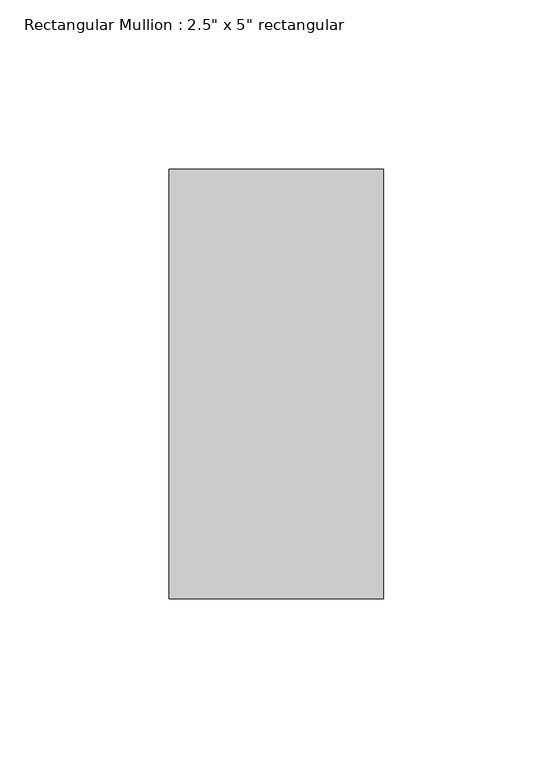
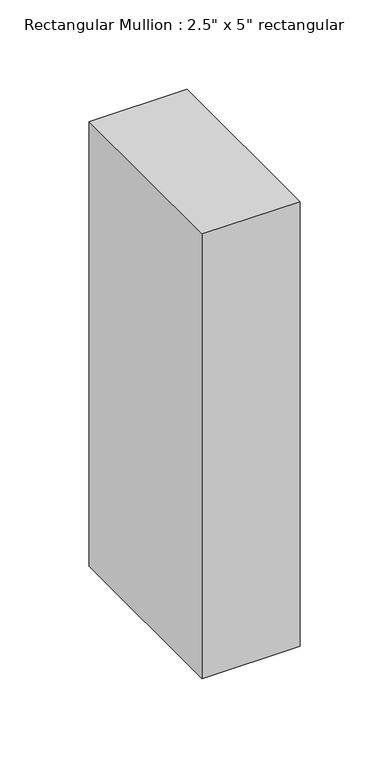
"""IFC4 building model written with IfcOpenShell, lengths in millimetres: member geometry."""

from ifc_helpers import new_model, si_unit, frame, origin, place, context, project, spatial, polyline, outline, extrude, source, transform, mapped, element, save


def member_3c3dc66a(model_context):
    return source(origin(), model_context, "Body", "SweptSolid", [
        extrude(outline(polyline([(0.0, 63.5), (0.0, -63.5), (-63.5, -63.5), (-63.5, 63.5), (0.0, 63.5)])), frame((0.0, 0.0, -304.8), z_axis=(0.0, 0.0, 1.0), x_axis=(1.0, 0.0, 0.0)), (0.0, 0.0, 1.0), 304.8),
    ])


if __name__ == "__main__":
    model = new_model("IFC4")
    model_context = context("Model", 3, world=origin())
    ifc_project = project(units=[si_unit("LENGTHUNIT", "METRE", prefix="MILLI")], contexts=[model_context])
    site = spatial("IfcSite", under=ifc_project)
    building = spatial("IfcBuilding", under=site)
    placement = place(None, origin())
    member_shape = member_3c3dc66a(model_context)
    element("IfcMember", 1, ObjectType="Rectangular Mullion : 2.5\" x 5\" rectangular", at=placement, inside=building, context=model_context, shape_type="MappedRepresentation", body=[
        mapped(member_shape, transform((0.0, 0.0, 0.0), x_axis=(1.0, 0.0, 0.0), y_axis=(0.0, 1.0, 0.0), z_axis=(0.0, 0.0, 1.0))),
    ])
    save(model, "model.ifc")

# Revit data of these elements
# Type "Rectangular Mullion : 2.5\" x 5\" rectangular"
#   built-in parameter 1007304 = 0.416667 (stored number, unit not read)
#   built-in parameter 1007301 = 0.104167 (stored number, unit not read)
#   built-in parameter 1007300 = 0.104167 (stored number, unit not read)
# Element 1 (IfcMember, "Rectangular Mullion : 2.5\" x 5\" rectangular")
#   Materials on its faces: "Iron, Ductile"
# Materials
#   "Iron, Ductile": class "Metal", colour RGB 0 0 0, transparency 0, Description = "Ductile cast iron", Cost = 0
